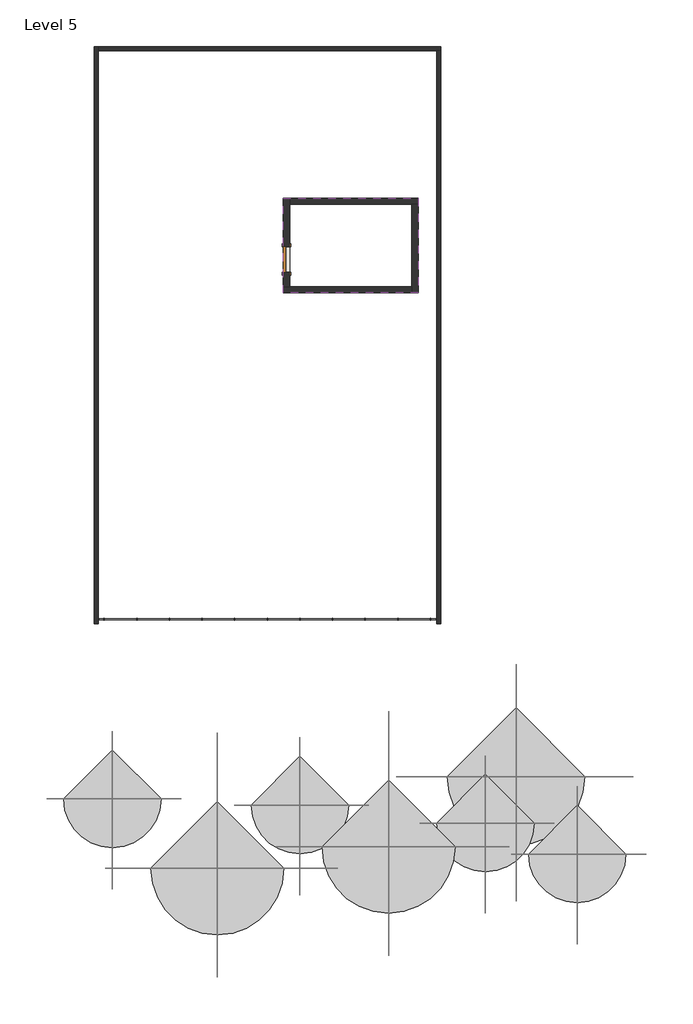
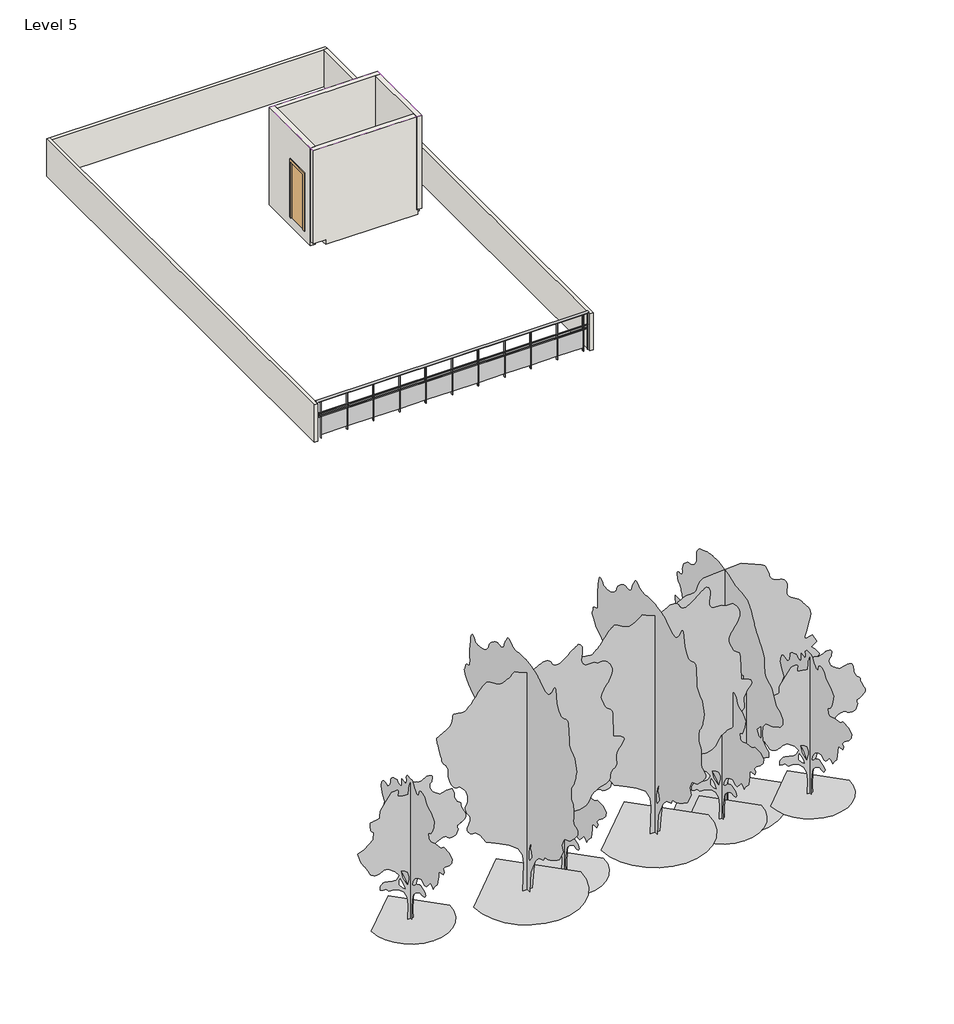
# One storey, incomplete: 7 geographic elements, 7 walls, 1 covering, 1 door, 1 railing.
"""IFC4 building model written with IfcOpenShell, lengths in millimetres."""

from ifc_helpers import new_model, si_unit, point, frame, origin, place, context, project, spatial, polyline, ellipse_curve, trimmed, outline, extrude, faceted_brep, transform, mapped, element, save
from ifc_brep_helpers import plane_surface, extruded_surface, advanced_brep
from components import door_57c759c4, rpc_tree_deciduous_honey_locust_25_cc46a1f1, rpc_tree_deciduous_japanese_cherry_15_e499737d, rpc_tree_deciduous_largetooth_aspen_25_f6cd7aa4

model = new_model("IFC4")

# Units and contexts
model_context = context("Model", 3, world=origin())
ifc_project = project(units=[si_unit("LENGTHUNIT", "METRE", prefix="MILLI")], contexts=[model_context])

# Site, building, storey
site = spatial("IfcSite", under=ifc_project)
building = spatial("IfcBuilding", under=site)
storey = spatial("IfcBuildingStorey", under=building, Name="Level 5", Elevation=12801.6)

# Covering
placement = place(None, origin())
element("IfcCovering", 1, ObjectType="2' x 4' ACT System", at=placement, inside=storey, context=model_context, shape_type="SweptSolid", body=[
    extrude(outline(polyline([(-1637.0893966, 3362.5242824), (1715.7106034, 3362.5242824), (1715.7106034, 1000.3242824), (-1637.0893966, 1000.3242824), (-1637.0893966, 3362.5242824)])), frame((0.0, 0.0, 16002.0), z_axis=(0.0, 0.0, 1.0), x_axis=(1.0, 0.0, 0.0)), (0.0, 0.0, 1.0), 57.15),
])

# Door
door_shape = door_57c759c4(model_context)
element("IfcDoor", 2, ObjectType="Single-Flush : 2'1\"", at=placement, inside=storey, context=model_context, shape_type="MappedRepresentation", body=[
    mapped(door_shape, transform((-1560.8893966, 1838.5242824, 13106.4), x_axis=(0.0, 1.0, 0.0), y_axis=(-1.0, 0.0, 0.0), z_axis=(0.0, 0.0, 1.0))),
])

# Geographic elements
rpc_tree_deciduous_honey_locust_25_shape = rpc_tree_deciduous_honey_locust_25_cc46a1f1(model_context)
element("IfcGeographicElement", 3, ObjectType="RPC Tree - Deciduous : Honey Locust - 25'", at=placement, inside=storey, context=model_context, shape_type="MappedRepresentation", body=[
    mapped(rpc_tree_deciduous_honey_locust_25_shape, transform((-3284.162336, -13331.4387628, 1075.0233882), x_axis=(1.0, 0.0, 0.0), y_axis=(0.0, 1.0, 0.0), z_axis=(0.0, 0.0, 1.0))),
])
element("IfcGeographicElement", 4, ObjectType="RPC Tree - Deciduous : Honey Locust - 25'", at=placement, inside=storey, context=model_context, shape_type="MappedRepresentation", body=[
    mapped(rpc_tree_deciduous_honey_locust_25_shape, transform((982.995052, -12793.8979314, 1125.9754113), x_axis=(1.0, 0.0, 0.0), y_axis=(0.0, 1.0, 0.0), z_axis=(0.0, 0.0, 1.0))),
])
rpc_tree_deciduous_japanese_cherry_15_shape = rpc_tree_deciduous_japanese_cherry_15_e499737d(model_context)
element("IfcGeographicElement", 5, ObjectType="RPC Tree - Deciduous : Japanese Cherry - 15'", at=placement, inside=storey, context=model_context, shape_type="MappedRepresentation", body=[
    mapped(rpc_tree_deciduous_japanese_cherry_15_shape, transform((-5900.364062, -11604.8142637, 0.0), x_axis=(1.0, 0.0, 0.0), y_axis=(0.0, 1.0, 0.0), z_axis=(0.0, 0.0, 1.0))),
])
element("IfcGeographicElement", 6, ObjectType="RPC Tree - Deciduous : Japanese Cherry - 15'", at=placement, inside=storey, context=model_context, shape_type="MappedRepresentation", body=[
    mapped(rpc_tree_deciduous_japanese_cherry_15_shape, transform((-1226.764062, -11757.2142637, 0.0), x_axis=(1.0, 0.0, 0.0), y_axis=(0.0, 1.0, 0.0), z_axis=(0.0, 0.0, 1.0))),
])
element("IfcGeographicElement", 7, ObjectType="RPC Tree - Deciduous : Japanese Cherry - 15'", at=placement, inside=storey, context=model_context, shape_type="MappedRepresentation", body=[
    mapped(rpc_tree_deciduous_japanese_cherry_15_shape, transform((5681.9840493, -12977.3814912, 880.3293818), x_axis=(1.0, 0.0, 0.0), y_axis=(0.0, 1.0, 0.0), z_axis=(0.0, 0.0, 1.0))),
])
element("IfcGeographicElement", 8, ObjectType="RPC Tree - Deciduous : Japanese Cherry - 15'", at=placement, inside=storey, context=model_context, shape_type="MappedRepresentation", body=[
    mapped(rpc_tree_deciduous_japanese_cherry_15_shape, transform((3395.9540849, -12207.2902913, 389.9234269), x_axis=(1.0, 0.0, 0.0), y_axis=(0.0, 1.0, 0.0), z_axis=(0.0, 0.0, 1.0))),
])
rpc_tree_deciduous_largetooth_aspen_25_shape = rpc_tree_deciduous_largetooth_aspen_25_f6cd7aa4(model_context)
element("IfcGeographicElement", 9, ObjectType="RPC Tree - Deciduous : Largetooth Aspen - 25'", at=placement, inside=storey, context=model_context, shape_type="MappedRepresentation", body=[
    mapped(rpc_tree_deciduous_largetooth_aspen_25_shape, transform((4158.035938, -11046.0142637, 0.0), x_axis=(1.0, 0.0, 0.0), y_axis=(0.0, 1.0, 0.0), z_axis=(0.0, 0.0, 1.0))),
])

# Railing
element("IfcRailing", 10, ObjectType="Glass Panel - Bottom Fill", at=placement, inside=storey, context=model_context, shape_type="SolidModel", body=[
    advanced_brep(
    [(2176.835938, -7172.5142637, 14325.6), (2176.835938, -7096.3142637, 14325.6), (-6255.964062, -7172.5142637, 14325.6), (-6255.964062, -7096.3142637, 14325.6)],
    [
        (0, 1, ellipse_curve(frame((2176.835938, -7134.4142637, 14325.6), z_axis=(1.0, 0.0, 0.0), x_axis=(0.0, 1.0, 0.0)), 38.1, 28.575)),
        (1, 0, ellipse_curve(frame((2176.835938, -7134.4142637, 14325.6), z_axis=(1.0, 0.0, 0.0), x_axis=(0.0, 1.0, 0.0)), 38.1, 28.575)),
        (2, 3, ellipse_curve(frame((-6255.964062, -7134.4142637, 14325.6), z_axis=(-1.0, 0.0, 0.0), x_axis=(0.0, 1.0, 0.0)), 38.1, 28.575)),
        (3, 2, ellipse_curve(frame((-6255.964062, -7134.4142637, 14325.6), z_axis=(-1.0, 0.0, 0.0), x_axis=(0.0, 1.0, 0.0)), 38.1, 28.575)),
        (0, 2),
        (3, 1),
    ],
    [
        plane_surface(frame((2176.835938, -7134.4142637, 14325.6), z_axis=(1.0, 0.0, 0.0), x_axis=(0.0, -1.0, 0.0))),
        plane_surface(frame((-6255.964062, -7134.4142637, 14325.6), z_axis=(-1.0, 0.0, 0.0), x_axis=(0.0, -1.0, 0.0))),
        extruded_surface(trimmed(ellipse_curve(frame((-6255.964062, -7134.4142637, 14325.6), z_axis=(1.0, 0.0, 0.0), x_axis=(0.0, 1.0, 0.0)), 38.1, 28.575), [point((-6255.964062, -7172.5142637, 14325.6))], [point((-6255.964062, -7096.3142637, 14325.6))], True, "CARTESIAN"), (8432.8, 0.0, 0.0), 8432.8),
        extruded_surface(trimmed(ellipse_curve(frame((-6255.964062, -7134.4142637, 14325.6), z_axis=(1.0, 0.0, 0.0), x_axis=(0.0, 1.0, 0.0)), 38.1, 28.575), [point((-6255.964062, -7096.3142637, 14325.6))], [point((-6255.964062, -7172.5142637, 14325.6))], True, "CARTESIAN"), (8432.8, 0.0, 0.0), 8432.8),
    ],
    [
        (0, [[1, 2]]),
        (1, [[3, 4]]),
        (2, [[-1, 5, -4, 6]]),
        (3, [[-2, -6, -3, -5]]),
    ],
),
    extrude(outline(polyline([(2176.835938, -7121.7142637), (2176.835938, -7147.1142637), (-6255.964062, -7147.1142637), (-6255.964062, -7121.7142637), (2176.835938, -7121.7142637)])), frame((0.0, 0.0, 13906.5), z_axis=(0.0, 0.0, 1.0), x_axis=(1.0, 0.0, 0.0)), (0.0, 0.0, 1.0), 25.4),
    extrude(outline(polyline([(2176.835938, -7121.7142637), (2176.835938, -7147.1142637), (-6255.964062, -7147.1142637), (-6255.964062, -7121.7142637), (2176.835938, -7121.7142637)])), frame((0.0, 0.0, 13804.9), z_axis=(0.0, 0.0, 1.0), x_axis=(1.0, 0.0, 0.0)), (0.0, 0.0, 1.0), 25.4),
    extrude(outline(polyline([(-6097.214062, -7109.0142637), (-6097.214062, -7159.8142637), (-6109.914062, -7159.8142637), (-6109.914062, -7109.0142637), (-6097.214062, -7109.0142637)])), frame((0.0, 0.0, 13106.4), z_axis=(0.0, 0.0, 1.0), x_axis=(1.0, 0.0, 0.0)), (0.0, 0.0, 1.0), 1190.625),
    extrude(outline(polyline([(-5290.764062, -7140.9494207), (-6103.564062, -7140.9494207), (-6103.564062, -7134.5994207), (-5290.764062, -7134.5994207), (-5290.764062, -7140.9494207)])), frame((0.0, 0.0, 13208.0), z_axis=(0.0, 0.0, 1.0), x_axis=(1.0, 0.0, 0.0)), (0.0, 0.0, 1.0), 596.9),
    extrude(outline(polyline([(-5284.414062, -7109.0142637), (-5284.414062, -7159.8142637), (-5297.114062, -7159.8142637), (-5297.114062, -7109.0142637), (-5284.414062, -7109.0142637)])), frame((0.0, 0.0, 13106.4), z_axis=(0.0, 0.0, 1.0), x_axis=(1.0, 0.0, 0.0)), (0.0, 0.0, 1.0), 1190.625),
    extrude(outline(polyline([(-4477.964062, -7140.9494207), (-5290.764062, -7140.9494207), (-5290.764062, -7134.5994207), (-4477.964062, -7134.5994207), (-4477.964062, -7140.9494207)])), frame((0.0, 0.0, 13208.0), z_axis=(0.0, 0.0, 1.0), x_axis=(1.0, 0.0, 0.0)), (0.0, 0.0, 1.0), 596.9),
    extrude(outline(polyline([(-4471.614062, -7109.0142637), (-4471.614062, -7159.8142637), (-4484.314062, -7159.8142637), (-4484.314062, -7109.0142637), (-4471.614062, -7109.0142637)])), frame((0.0, 0.0, 13106.4), z_axis=(0.0, 0.0, 1.0), x_axis=(1.0, 0.0, 0.0)), (0.0, 0.0, 1.0), 1190.625),
    extrude(outline(polyline([(-3665.164062, -7140.9494207), (-4477.964062, -7140.9494207), (-4477.964062, -7134.5994207), (-3665.164062, -7134.5994207), (-3665.164062, -7140.9494207)])), frame((0.0, 0.0, 13208.0), z_axis=(0.0, 0.0, 1.0), x_axis=(1.0, 0.0, 0.0)), (0.0, 0.0, 1.0), 596.9),
    extrude(outline(polyline([(-3658.814062, -7109.0142637), (-3658.814062, -7159.8142637), (-3671.514062, -7159.8142637), (-3671.514062, -7109.0142637), (-3658.814062, -7109.0142637)])), frame((0.0, 0.0, 13106.4), z_axis=(0.0, 0.0, 1.0), x_axis=(1.0, 0.0, 0.0)), (0.0, 0.0, 1.0), 1190.625),
    extrude(outline(polyline([(-2852.364062, -7140.9494207), (-3665.164062, -7140.9494207), (-3665.164062, -7134.5994207), (-2852.364062, -7134.5994207), (-2852.364062, -7140.9494207)])), frame((0.0, 0.0, 13208.0), z_axis=(0.0, 0.0, 1.0), x_axis=(1.0, 0.0, 0.0)), (0.0, 0.0, 1.0), 596.9),
    extrude(outline(polyline([(-2846.014062, -7109.0142637), (-2846.014062, -7159.8142637), (-2858.714062, -7159.8142637), (-2858.714062, -7109.0142637), (-2846.014062, -7109.0142637)])), frame((0.0, 0.0, 13106.4), z_axis=(0.0, 0.0, 1.0), x_axis=(1.0, 0.0, 0.0)), (0.0, 0.0, 1.0), 1190.625),
    extrude(outline(polyline([(-2039.564062, -7140.9494207), (-2852.364062, -7140.9494207), (-2852.364062, -7134.5994207), (-2039.564062, -7134.5994207), (-2039.564062, -7140.9494207)])), frame((0.0, 0.0, 13208.0), z_axis=(0.0, 0.0, 1.0), x_axis=(1.0, 0.0, 0.0)), (0.0, 0.0, 1.0), 596.9),
    extrude(outline(polyline([(-2033.214062, -7109.0142637), (-2033.214062, -7159.8142637), (-2045.914062, -7159.8142637), (-2045.914062, -7109.0142637), (-2033.214062, -7109.0142637)])), frame((0.0, 0.0, 13106.4), z_axis=(0.0, 0.0, 1.0), x_axis=(1.0, 0.0, 0.0)), (0.0, 0.0, 1.0), 1190.625),
    extrude(outline(polyline([(-1226.764062, -7140.9494207), (-2039.564062, -7140.9494207), (-2039.564062, -7134.5994207), (-1226.764062, -7134.5994207), (-1226.764062, -7140.9494207)])), frame((0.0, 0.0, 13208.0), z_axis=(0.0, 0.0, 1.0), x_axis=(1.0, 0.0, 0.0)), (0.0, 0.0, 1.0), 596.9),
    extrude(outline(polyline([(-1220.414062, -7109.0142637), (-1220.414062, -7159.8142637), (-1233.114062, -7159.8142637), (-1233.114062, -7109.0142637), (-1220.414062, -7109.0142637)])), frame((0.0, 0.0, 13106.4), z_axis=(0.0, 0.0, 1.0), x_axis=(1.0, 0.0, 0.0)), (0.0, 0.0, 1.0), 1190.625),
    extrude(outline(polyline([(-413.964062, -7140.9494207), (-1226.764062, -7140.9494207), (-1226.764062, -7134.5994207), (-413.964062, -7134.5994207), (-413.964062, -7140.9494207)])), frame((0.0, 0.0, 13208.0), z_axis=(0.0, 0.0, 1.0), x_axis=(1.0, 0.0, 0.0)), (0.0, 0.0, 1.0), 596.9),
    extrude(outline(polyline([(-407.614062, -7109.0142637), (-407.614062, -7159.8142637), (-420.314062, -7159.8142637), (-420.314062, -7109.0142637), (-407.614062, -7109.0142637)])), frame((0.0, 0.0, 13106.4), z_axis=(0.0, 0.0, 1.0), x_axis=(1.0, 0.0, 0.0)), (0.0, 0.0, 1.0), 1190.625),
    extrude(outline(polyline([(398.835938, -7140.9494207), (-413.964062, -7140.9494207), (-413.964062, -7134.5994207), (398.835938, -7134.5994207), (398.835938, -7140.9494207)])), frame((0.0, 0.0, 13208.0), z_axis=(0.0, 0.0, 1.0), x_axis=(1.0, 0.0, 0.0)), (0.0, 0.0, 1.0), 596.9),
    extrude(outline(polyline([(405.185938, -7109.0142637), (405.185938, -7159.8142637), (392.485938, -7159.8142637), (392.485938, -7109.0142637), (405.185938, -7109.0142637)])), frame((0.0, 0.0, 13106.4), z_axis=(0.0, 0.0, 1.0), x_axis=(1.0, 0.0, 0.0)), (0.0, 0.0, 1.0), 1190.625),
    extrude(outline(polyline([(1211.635938, -7140.9494207), (398.835938, -7140.9494207), (398.835938, -7134.5994207), (1211.635938, -7134.5994207), (1211.635938, -7140.9494207)])), frame((0.0, 0.0, 13208.0), z_axis=(0.0, 0.0, 1.0), x_axis=(1.0, 0.0, 0.0)), (0.0, 0.0, 1.0), 596.9),
    extrude(outline(polyline([(1217.985938, -7109.0142637), (1217.985938, -7159.8142637), (1205.285938, -7159.8142637), (1205.285938, -7109.0142637), (1217.985938, -7109.0142637)])), frame((0.0, 0.0, 13106.4), z_axis=(0.0, 0.0, 1.0), x_axis=(1.0, 0.0, 0.0)), (0.0, 0.0, 1.0), 1190.625),
    extrude(outline(polyline([(2024.435938, -7140.9494207), (1211.635938, -7140.9494207), (1211.635938, -7134.5994207), (2024.435938, -7134.5994207), (2024.435938, -7140.9494207)])), frame((0.0, 0.0, 13208.0), z_axis=(0.0, 0.0, 1.0), x_axis=(1.0, 0.0, 0.0)), (0.0, 0.0, 1.0), 596.9),
    extrude(outline(polyline([(2030.785938, -7109.0142637), (2030.785938, -7159.8142637), (2018.085938, -7159.8142637), (2018.085938, -7109.0142637), (2030.785938, -7109.0142637)])), frame((0.0, 0.0, 13106.4), z_axis=(0.0, 0.0, 1.0), x_axis=(1.0, 0.0, 0.0)), (0.0, 0.0, 1.0), 1190.625),
    extrude(outline(polyline([(-6243.264062, -7124.8892637), (-6243.264062, -7143.9392637), (-6262.314062, -7143.9392637), (-6262.314062, -7124.8892637), (-6243.264062, -7124.8892637)])), frame((0.0, 0.0, 13106.4), z_axis=(0.0, 0.0, 1.0), x_axis=(1.0, 0.0, 0.0)), (0.0, 0.0, 1.0), 1190.625),
    extrude(outline(polyline([(2183.185938, -7124.8892637), (2183.185938, -7143.9392637), (2164.135938, -7143.9392637), (2164.135938, -7124.8892637), (2183.185938, -7124.8892637)])), frame((0.0, 0.0, 13106.4), z_axis=(0.0, 0.0, 1.0), x_axis=(1.0, 0.0, 0.0)), (0.0, 0.0, 1.0), 1190.625),
])

# Walls
element("IfcWall", 11, ObjectType="Generic - 4\"", at=placement, inside=storey, context=model_context, shape_type="Brep", body=[
    faceted_brep([(2278.435938, 7140.3857363, 13106.4), (-6255.964062, 7140.3857363, 13106.4), (-6255.964062, 7140.3857363, 14325.6), (2278.435938, 7140.3857363, 14325.6), (2278.435938, 7038.7857363, 13106.4), (2278.435938, 7038.7857363, 14325.6), (2176.835938, 7038.7857363, 14325.6), (-6255.964062, 7038.7857363, 14325.6), (-6255.964062, 7038.7857363, 13106.4), (2176.835938, 7038.7857363, 13106.4)], [[[0, 1, 2, 3]], [[4, 5, 6, 7, 8, 9]], [[1, 0, 4, 9, 8]], [[3, 2, 7, 6, 5]], [[0, 3, 5, 4]], [[2, 1, 8, 7]]]),
])
element("IfcWall", 12, ObjectType="Generic - 4\"", at=placement, inside=storey, context=model_context, shape_type="SweptSolid", body=[
    extrude(outline(polyline([(2278.435938, 7038.7857363), (2278.435938, -7236.0142637), (2176.835938, -7236.0142637), (2176.835938, 7038.7857363), (2278.435938, 7038.7857363)])), frame((0.0, 0.0, 13106.4), z_axis=(0.0, 0.0, 1.0), x_axis=(1.0, 0.0, 0.0)), (0.0, 0.0, 1.0), 1219.2),
])
element("IfcWall", 13, ObjectType="Generic - 4\"", at=placement, inside=storey, context=model_context, shape_type="Brep", body=[
    faceted_brep([(-6357.564062, 7140.3857363, 13106.4), (-6357.564062, -7236.0142637, 13106.4), (-6357.564062, -7236.0142637, 14325.6), (-6357.564062, 7140.3857363, 14325.6), (-6255.964062, 7140.3857363, 13106.4), (-6255.964062, 7140.3857363, 14325.6), (-6255.964062, 7038.7857363, 14325.6), (-6255.964062, -7236.0142637, 14325.6), (-6255.964062, -7236.0142637, 13106.4), (-6255.964062, 7038.7857363, 13106.4)], [[[0, 1, 2, 3]], [[4, 5, 6, 7, 8, 9]], [[1, 0, 4, 9, 8]], [[2, 1, 8, 7]], [[3, 2, 7, 6, 5]], [[0, 3, 5, 4]]]),
])
element("IfcWall", 14, ObjectType="Generic - 6\"", at=placement, inside=storey, context=model_context, shape_type="Brep", body=[
    faceted_brep([(-1252.164062, 1000.3242824, 12801.6), (1592.635938, 1000.3242824, 12801.6), (1592.635938, 1000.3242824, 12954.0), (1563.3106034, 1000.3242824, 12954.0), (1563.3106034, 1000.3242824, 16002.0), (-1637.0893966, 1000.3242824, 16002.0), (-1637.0893966, 1000.3242824, 12954.0), (-1252.164062, 1000.3242824, 12954.0), (-1252.164062, 1152.7242824, 12801.6), (-1252.164062, 1152.7242824, 12954.0), (-1637.0893966, 1152.7242824, 12954.0), (-1637.0893966, 1152.7242824, 16002.0), (-1484.6893966, 1152.7242824, 16002.0), (1563.3106034, 1152.7242824, 16002.0), (1563.3106034, 1152.7242824, 12954.0), (1592.635938, 1152.7242824, 12954.0), (1592.635938, 1152.7242824, 12801.6), (1563.3106034, 1120.5857363, 12954.0), (1592.635938, 1044.3857363, 12954.0)], [[[0, 1, 2, 3, 4, 5, 6, 7]], [[8, 9, 10, 11, 12, 13, 14, 15, 16]], [[1, 0, 8, 16]], [[5, 4, 13, 12, 11]], [[6, 10, 9, 7]], [[0, 7, 9, 8]], [[6, 5, 11, 10]], [[14, 17, 3, 2, 18, 15]], [[2, 1, 16, 15, 18]], [[4, 3, 17, 14, 13]]]),
])
element("IfcWall", 15, ObjectType="Generic - 6\"", at=placement, inside=storey, context=model_context, shape_type="Brep", body=[
    faceted_brep([(-1637.0893966, 3362.5242824, 12801.6), (-1637.0893966, 1152.7242824, 12801.6), (-1637.0893966, 1152.7242824, 12954.0), (-1637.0893966, 1152.7242824, 16002.0), (-1637.0893966, 3362.5242824, 16002.0), (-1637.0893966, 1521.0242824, 13106.4), (-1637.0893966, 2156.0242824, 13106.4), (-1637.0893966, 2156.0242824, 14935.2), (-1637.0893966, 1521.0242824, 14935.2), (-1484.6893966, 3362.5242824, 12801.6), (-1484.6893966, 3362.5242824, 16002.0), (-1484.6893966, 3210.1242824, 16002.0), (-1484.6893966, 1152.7242824, 16002.0), (-1484.6893966, 1152.7242824, 12801.6), (-1484.6893966, 3210.1242824, 12801.6), (-1484.6893966, 1521.0242824, 13106.4), (-1484.6893966, 1521.0242824, 14935.2), (-1484.6893966, 2156.0242824, 14935.2), (-1484.6893966, 2156.0242824, 13106.4)], [[[0, 1, 2, 3, 4], [5, 6, 7, 8]], [[9, 10, 11, 12, 13, 14], [15, 16, 17, 18]], [[1, 0, 9, 14, 13]], [[4, 3, 12, 11, 10]], [[0, 4, 10, 9]], [[3, 2, 1, 13, 12]], [[6, 5, 15, 18]], [[7, 6, 18, 17]], [[8, 7, 17, 16]], [[5, 8, 16, 15]]]),
])
element("IfcWall", 16, ObjectType="Generic - 6\"", at=placement, inside=storey, context=model_context, shape_type="Brep", body=[
    faceted_brep([(1592.635938, 3362.5242824, 12801.6), (-1484.6893966, 3362.5242824, 12801.6), (-1484.6893966, 3362.5242824, 16002.0), (1715.7106034, 3362.5242824, 16002.0), (1715.7106034, 3362.5242824, 12954.0), (1592.635938, 3362.5242824, 12954.0), (1592.635938, 3210.1242824, 12801.6), (1592.635938, 3210.1242824, 12954.0), (1715.7106034, 3210.1242824, 12954.0), (1715.7106034, 3210.1242824, 16002.0), (1563.3106034, 3210.1242824, 16002.0), (-1484.6893966, 3210.1242824, 16002.0), (-1484.6893966, 3210.1242824, 12801.6), (1715.7106034, 3254.1857363, 12954.0), (1592.635938, 3330.3857363, 12954.0)], [[[0, 1, 2, 3, 4, 5]], [[6, 7, 8, 9, 10, 11, 12]], [[1, 0, 6, 12]], [[3, 2, 11, 10, 9]], [[2, 1, 12, 11]], [[4, 13, 8, 7, 14, 5]], [[0, 5, 14, 7, 6]], [[4, 3, 9, 8, 13]]]),
])
element("IfcWall", 17, ObjectType="Generic - 6\"", at=placement, inside=storey, context=model_context, shape_type="Brep", body=[
    faceted_brep([(1715.7106034, 1120.5857363, 12801.6), (1715.7106034, 3254.1857363, 12801.6), (1715.7106034, 3254.1857363, 12954.0), (1715.7106034, 3210.1242824, 12954.0), (1715.7106034, 3210.1242824, 16002.0), (1715.7106034, 1000.3242824, 16002.0), (1715.7106034, 1000.3242824, 12954.0), (1715.7106034, 1120.5857363, 12954.0), (1563.3106034, 1120.5857363, 12801.6), (1563.3106034, 1120.5857363, 12954.0), (1563.3106034, 1000.3242824, 12954.0), (1563.3106034, 1000.3242824, 16002.0), (1563.3106034, 1152.7242824, 16002.0), (1563.3106034, 3210.1242824, 16002.0), (1563.3106034, 3210.1242824, 12954.0), (1563.3106034, 3254.1857363, 12954.0), (1563.3106034, 3254.1857363, 12801.6), (1592.635938, 3210.1242824, 12954.0), (1592.635938, 3254.1857363, 12954.0), (1592.635938, 1000.3242824, 12954.0), (1592.635938, 1120.5857363, 12954.0)], [[[0, 1, 2, 3, 4, 5, 6, 7]], [[8, 9, 10, 11, 12, 13, 14, 15, 16]], [[1, 0, 8, 16]], [[5, 4, 13, 12, 11]], [[14, 17, 3, 2, 18, 15]], [[2, 1, 16, 15, 18]], [[4, 3, 17, 14, 13]], [[6, 19, 10, 9, 20, 7]], [[0, 7, 20, 9, 8]], [[6, 5, 11, 10, 19]]]),
])

save(model, "model.ifc")

# Revit data of these elements
# Type "2' x 4' ACT System"
#   Assembly Code = "C3030210"
#   built-in parameter 1002203 = 1 (stored number, unit not read)
#   built-in parameter 1002202 = 1 (stored number, unit not read)
#   Layers, outside or top first: 0' - 1 5/8" "Default" (function 1); 0' - 0 5/8" "Acoustic Ceiling Tile 24 x 48" (function 5)
# Type "Single-Flush : 2'1\""
#   Type Mark = "9"
#   Construction Type Id = "MDOOR"
#   Assembly Code = "C1020"
#   Analytic Construction = "Metal"
#   Thickness = 0' - 2"
#   Heat Transfer Coefficient (U) = 0.651978 BTU/(h·ft²·°F)
#   Height = 6' - 0"
#   Trim Projection Ext = 0' - 1"
#   Trim Projection Int = 0' - 1"
#   Trim Width = 0' - 3"
#   Width = 2' - 1"
#   Define Thermal Properties by = 1
#   Door Material = Door - Panel
#   Frame Material = Door - Frame
#   Visual Light Transmittance = 0
#   Solar Heat Gain Coefficient = 0
#   Function = (empty or 0)
#   Wall Closure = (empty or 0)
# Type "RPC Tree - Deciduous : Honey Locust - 25'"
#   built-in parameter 1005198 = "{2, 15},{39, RPC-16-G2VH-N100-5X50-0000-ST1L-LVER-AU},{1, 0},{1, 0},{2, 35},{1, 8},{5, Color},{1, 0},{1, 0},{3, 0.8},{3, 0.8},{3, 0.8},{1, 8},{7, BBoxMin},{1, 0},{1, 0},{1, 0},{1, 0},{1, 0},{1, 8},{7, BBoxMax},{1, 0},{1, 0},{1, 0},{1, 0},{1, 0},{2, 11},{9, RPCTypeId},{1, 0},{1, 0},{39, RPC-16-G2VH-N100-5X50-0000-ST1L-LVER-AU},{1, 6},{14, RPCPlantHeight},{1, 0},{1, 0},{2, 25},{2, 11},{7, keyword},{1, 0},{1, 0},{224, :Geometry:RPC:Honey-Locust:Gleditsia triacanthos L.  Rare in Canada; occurs in southwestern Ontario; commonly planted beyond its range because of its tolerance to droughty and alkaline soils; frequently becoming naturalized.},{2, 11},{8, category},{1, 0},{1, 0},{16, :Trees [General]},{2, 11},{12, LocalizedUID},{1, 0},{1, 0},{12, Honey-Locust},{2, 14},{6, Height},{1, 0},{1, 0},{2, 25},{1, 2},{16, Cast Reflections},{1, 0},{1, 0},{1, 0},{1, 2},{12, Cast Shadows},{1, 0},{1, 0},{1, 1},{1, 2},{9, Lock View},{1, 0},{1, 0},{1, 0},{1, 4},{5, ViewC},{1, 0},{1, 0},{1, 0},{2, 11},{20, AdvancedUIDefinition},{1, 0},{1, 0},{0, },{2, 11},{10, AssetLibID},{1, 0},{1, 0},{36, 4D3F6E72-3F99-4203-98E9-AF80B3C7A7A4},{2, 11},{10, BaseSchema},{1, 0},{1, 0},{9, RPCSchema},{2, 11},{12, ExchangeGUID},{1, 0},{1, 0},{0, },{1, 2},{6, Hidden},{1, 0},{1, 0},{1, 0},{1, 4},{11, RPCCategory},{1, 0},{1, 0},{1, 0},{2, 11},{8, RPCImage},{1, 0},{1, 0},{0, },{1, 4},{13, SchemaVersion},{1, 0},{1, 0},{1, 4},{2, 11},{12, UIDefinition},{1, 0},{1, 0},{0, },{2, 11},{6, UIName},{1, 0},{1, 0},{39, RPC-16-G2VH-N100-5X50-0000-ST1L-LVER-AU},{2, 11},{11, VersionGUID},{1, 0},{1, 0},{9, RPCSchema},{2, 11},{9, assettype},{1, 0},{1, 0},{11, RPCGeometry},{2, 11},{11, description},{1, 0},{1, 0},{0, },{2, 11},{9, localname},{1, 0},{1, 0},{3, RPC},{2, 11},{9, localtype},{1, 0},{1, 0},{3, RPC},{1, 4},{8, revision},{1, 0},{1, 0},{1, 1},{2, 11},{9, thumbnail},{1, 0},{1, 0},{0, },{1, 4},{7, version},{1, 0},{1, 0},{1, 1},{1, 2},{20, RPC_Cast Reflections},{1, 0},{1, 0},{1, 1},{1, 2},{16, RPC_Cast Shadows},{1, 0},{1, 0},{1, 1},{1, 2},{13, RPC_Lock View},{1, 0},{1, 0},{1, 0},{1, 4},{9, RPC_ViewC},{1, 0},{1, 0},{1, 0},{21, assetlibrary_base.fbx},{1, 5},"
#   built-in parameter 1005195 = "RPC-16-G2VH-N100-5X50-0000-ST1L-LVER-AU"
#   Type Comments = "Honey Locust"
#   Assembly Code = "G2050500"
#   Height = 25' - 0"
#   Default Elevation = 0
# Type "RPC Tree - Deciduous : Japanese Cherry - 15'"
#   built-in parameter 1005198 = "{2, 15},{39, RPC-16-FXGW-2MQ0-PN7K-A000-ST1L-LVER-AU},{1, 0},{1, 0},{2, 35},{1, 8},{5, Color},{1, 0},{1, 0},{3, 0.8},{3, 0.8},{3, 0.8},{1, 8},{7, BBoxMin},{1, 0},{1, 0},{1, 0},{1, 0},{1, 0},{1, 8},{7, BBoxMax},{1, 0},{1, 0},{1, 0},{1, 0},{1, 0},{2, 11},{9, RPCTypeId},{1, 0},{1, 0},{39, RPC-16-FXGW-2MQ0-PN7K-A000-ST1L-LVER-AU},{1, 6},{14, RPCPlantHeight},{1, 0},{1, 0},{2, 15},{2, 11},{7, keyword},{1, 0},{1, 0},{207, :Geometry:RPC:Japanese Flowering Cherry:Prunus serrulata Lindl:A landscape tree:valued for its abundant showy flowers; native to China and Japan.  Hardy only in the mildest parts of Canada and farther south.},{2, 11},{8, category},{1, 0},{1, 0},{16, :Trees [General]},{2, 11},{12, LocalizedUID},{1, 0},{1, 0},{25, Japanese Flowering Cherry},{2, 14},{6, Height},{1, 0},{1, 0},{2, 15},{1, 2},{16, Cast Reflections},{1, 0},{1, 0},{1, 0},{1, 2},{12, Cast Shadows},{1, 0},{1, 0},{1, 1},{1, 2},{9, Lock View},{1, 0},{1, 0},{1, 0},{1, 4},{5, ViewC},{1, 0},{1, 0},{1, 0},{2, 11},{20, AdvancedUIDefinition},{1, 0},{1, 0},{0, },{2, 11},{10, AssetLibID},{1, 0},{1, 0},{36, 4D3F6E72-3F99-4203-98E9-AF80B3C7A7A4},{2, 11},{10, BaseSchema},{1, 0},{1, 0},{9, RPCSchema},{2, 11},{12, ExchangeGUID},{1, 0},{1, 0},{0, },{1, 2},{6, Hidden},{1, 0},{1, 0},{1, 0},{1, 4},{11, RPCCategory},{1, 0},{1, 0},{1, 0},{2, 11},{8, RPCImage},{1, 0},{1, 0},{0, },{1, 4},{13, SchemaVersion},{1, 0},{1, 0},{1, 4},{2, 11},{12, UIDefinition},{1, 0},{1, 0},{0, },{2, 11},{6, UIName},{1, 0},{1, 0},{39, RPC-16-FXGW-2MQ0-PN7K-A000-ST1L-LVER-AU},{2, 11},{11, VersionGUID},{1, 0},{1, 0},{9, RPCSchema},{2, 11},{9, assettype},{1, 0},{1, 0},{11, RPCGeometry},{2, 11},{11, description},{1, 0},{1, 0},{0, },{2, 11},{9, localname},{1, 0},{1, 0},{3, RPC},{2, 11},{9, localtype},{1, 0},{1, 0},{3, RPC},{1, 4},{8, revision},{1, 0},{1, 0},{1, 1},{2, 11},{9, thumbnail},{1, 0},{1, 0},{0, },{1, 4},{7, version},{1, 0},{1, 0},{1, 1},{1, 2},{20, RPC_Cast Reflections},{1, 0},{1, 0},{1, 1},{1, 2},{16, RPC_Cast Shadows},{1, 0},{1, 0},{1, 1},{1, 2},{13, RPC_Lock View},{1, 0},{1, 0},{1, 0},{1, 4},{9, RPC_ViewC},{1, 0},{1, 0},{1, 0},{21, assetlibrary_base.fbx},{1, 5},"
#   built-in parameter 1005195 = "RPC-16-FXGW-2MQ0-PN7K-A000-ST1L-LVER-AU"
#   Type Comments = "Japanese Cherry"
#   Assembly Code = "G2050500"
#   Height = 15' - 0"
#   Default Elevation = 0
# Type "RPC Tree - Deciduous : Largetooth Aspen - 25'"
#   built-in parameter 1005198 = "{2, 15},{39, RPC-16-G0VG-J3PX-MQ0P-J000-ST1L-LVER-AU},{1, 0},{1, 0},{2, 35},{1, 8},{5, Color},{1, 0},{1, 0},{3, 0.8},{3, 0.8},{3, 0.8},{1, 8},{7, BBoxMin},{1, 0},{1, 0},{1, 0},{1, 0},{1, 0},{1, 8},{7, BBoxMax},{1, 0},{1, 0},{1, 0},{1, 0},{1, 0},{2, 11},{9, RPCTypeId},{1, 0},{1, 0},{39, RPC-16-G0VG-J3PX-MQ0P-J000-ST1L-LVER-AU},{1, 6},{14, RPCPlantHeight},{1, 0},{1, 0},{2, 25},{2, 11},{7, keyword},{1, 0},{1, 0},{178, :Geometry:RPC:Largetooth Aspen:Populus grandidentata:similar in form and aspect to trembling aspen; range does not extend as far west:east:or north; usually found on drier sites.},{2, 11},{8, category},{1, 0},{1, 0},{16, :Trees [General]},{2, 11},{12, LocalizedUID},{1, 0},{1, 0},{16, Largetooth Aspen},{2, 14},{6, Height},{1, 0},{1, 0},{2, 25},{1, 2},{16, Cast Reflections},{1, 0},{1, 0},{1, 0},{1, 2},{12, Cast Shadows},{1, 0},{1, 0},{1, 1},{1, 2},{9, Lock View},{1, 0},{1, 0},{1, 0},{1, 4},{5, ViewC},{1, 0},{1, 0},{1, 0},{2, 11},{20, AdvancedUIDefinition},{1, 0},{1, 0},{0, },{2, 11},{10, AssetLibID},{1, 0},{1, 0},{36, 4D3F6E72-3F99-4203-98E9-AF80B3C7A7A4},{2, 11},{10, BaseSchema},{1, 0},{1, 0},{9, RPCSchema},{2, 11},{12, ExchangeGUID},{1, 0},{1, 0},{0, },{1, 2},{6, Hidden},{1, 0},{1, 0},{1, 0},{1, 4},{11, RPCCategory},{1, 0},{1, 0},{1, 0},{2, 11},{8, RPCImage},{1, 0},{1, 0},{0, },{1, 4},{13, SchemaVersion},{1, 0},{1, 0},{1, 4},{2, 11},{12, UIDefinition},{1, 0},{1, 0},{0, },{2, 11},{6, UIName},{1, 0},{1, 0},{39, RPC-16-G0VG-J3PX-MQ0P-J000-ST1L-LVER-AU},{2, 11},{11, VersionGUID},{1, 0},{1, 0},{9, RPCSchema},{2, 11},{9, assettype},{1, 0},{1, 0},{11, RPCGeometry},{2, 11},{11, description},{1, 0},{1, 0},{0, },{2, 11},{9, localname},{1, 0},{1, 0},{3, RPC},{2, 11},{9, localtype},{1, 0},{1, 0},{3, RPC},{1, 4},{8, revision},{1, 0},{1, 0},{1, 1},{2, 11},{9, thumbnail},{1, 0},{1, 0},{0, },{1, 4},{7, version},{1, 0},{1, 0},{1, 1},{1, 2},{20, RPC_Cast Reflections},{1, 0},{1, 0},{1, 1},{1, 2},{16, RPC_Cast Shadows},{1, 0},{1, 0},{1, 1},{1, 2},{13, RPC_Lock View},{1, 0},{1, 0},{1, 0},{1, 4},{9, RPC_ViewC},{1, 0},{1, 0},{1, 0},{21, assetlibrary_base.fbx},{1, 5},"
#   built-in parameter 1005195 = "RPC-16-G0VG-J3PX-MQ0P-J000-ST1L-LVER-AU"
#   Type Comments = "Largetooth Aspen"
#   Assembly Code = "G2050500"
#   Height = 25' - 0"
#   Default Elevation = 0
# Type "Glass Panel - Bottom Fill"
#   Assembly Code = "C2010400"
#   built-in parameter 1008612 = 0.0416667 (stored number, unit not read)
#   built-in parameter 1008611 = 0.0416667 (stored number, unit not read)
#   built-in parameter 1008609 = 0.333333 (stored number, unit not read)
#   built-in parameter 1008604 = 0.166667 (stored number, unit not read)
#   built-in parameter 1008603 = 0.166667 (stored number, unit not read)
#   Railing Height = 4' - 0"
#   built-in parameter 1008630 = 2
#   built-in parameter 1008610 = 2
#   built-in parameter 1008618 = Baluster - Square : 3/4"
# Type "Generic - 4\""
#   Assembly Code = "B2010"
#   Layers, outside or top first: 0' - 4" no material (function 1)
# Type "Generic - 6\""
#   Assembly Code = "B2010"
#   Layers, outside or top first: 0' - 6" no material (function 1)
# Element 1 (IfcCovering, "2' x 4' ACT System")
#   Height Offset From Level = 10' - 6"
#   Phase Created = New Construction
#   Materials on its faces: "LAVENDER WHITE"
# Element 2 (IfcDoor, "Single-Flush : 2'1\"")
#   Phase Created = New Construction
#   Materials on its faces: "Door - Frame", "Door - Panel"
# Elements 3, 4 (IfcGeographicElement, "RPC Tree - Deciduous : Honey Locust - 25'")
#   Phase Created = New Construction
# Elements 5, 6, 7, 8 (IfcGeographicElement, "RPC Tree - Deciduous : Japanese Cherry - 15'")
#   Phase Created = New Construction
# Element 9 (IfcGeographicElement, "RPC Tree - Deciduous : Largetooth Aspen - 25'")
#   Phase Created = New Construction
# Element 10 (IfcRailing, "Glass Panel - Bottom Fill")
#   built-in parameter 1008621 = 1 (stored number, unit not read)
#   Phase Created = New Construction
#   Materials on its faces: "Glass"
# Elements 11, 12, 13 (IfcWall, "Generic - 4\"")
#   built-in parameter 1001111 = 1' - 0"
#   Top Offset = 0' - 0"
#   Base Offset = 1' - 0"
#   Unconnected Height = 4' - 0"
#   wall height = 4' - 0"
#   Phase Created = New Construction
#   Base Constraint = Level 5
#   Materials on its faces: "LAVENDER WHITE", "Default Wall"
# Elements 14, 15, 16, 17 (IfcWall, "Generic - 6\"")
#   Top Offset = 0' - 0"
#   Base Offset = 0' - 0"
#   Unconnected Height = 10' - 6"
#   wall height = 10' - 6"
#   Phase Created = New Construction
#   Base Constraint = Level 5
#   Materials on its faces: "Default Wall"
# Materials
#   "Default": colour RGB 127 127 127, transparency 0, Cost = 0
#   "Acoustic Ceiling Tile 24 x 48": class "Generic", colour RGB 229 229 229, transparency 0, Description = "Acoustic Ceiling Tile 24 x 48", Cost = 0
#   "Door - Panel": class "Wood", colour RGB 210 159 95, transparency 0, Cost = 0
#   "Door - Frame": colour RGB 118 70 51, transparency 0, Cost = 0
#   "LAVENDER WHITE": class "Generic", colour RGB 120 120 120, transparency 0, Cost = 0
#   "Glass": class "Glass", colour RGB 0 128 192, transparency 0.75, Description = "Soda Lime Glass", Cost = 0
#   "Default Wall": colour RGB 128 128 128, transparency 0, Cost = 0
